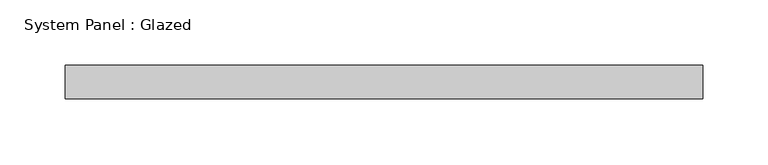
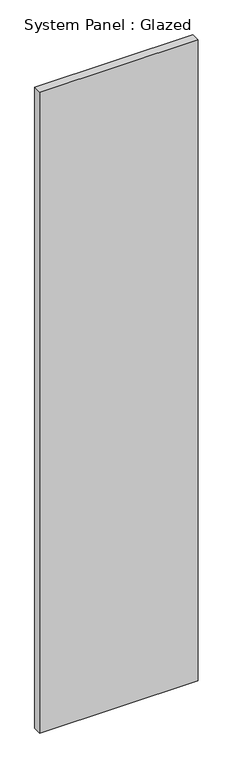
"""IFC4 building model written with IfcOpenShell, lengths in millimetres: plate geometry, System Panel : Glazed."""

from ifc_helpers import new_model, si_unit, origin, origin_with_axes, place, context, project, spatial, polyline, outline, extrude, source, transform, mapped, element, save


def system_panel_glazed_5e4042f1(model_context):
    return source(origin(), model_context, "Body", "SweptSolid", [
        extrude(outline(polyline([(243.5110562, -44.45), (-243.5110562, -44.45), (-243.5110562, -19.05), (243.5110562, -19.05), (243.5110562, -44.45)])), origin_with_axes(), (0.0, 0.0, 1.0), 2082.8),
    ])


if __name__ == "__main__":
    model = new_model("IFC4")
    model_context = context("Model", 3, world=origin())
    ifc_project = project(units=[si_unit("LENGTHUNIT", "METRE", prefix="MILLI")], contexts=[model_context])
    site = spatial("IfcSite", under=ifc_project)
    building = spatial("IfcBuilding", under=site)
    placement = place(None, origin())
    system_panel_glazed_shape = system_panel_glazed_5e4042f1(model_context)
    element("IfcPlate", 1, ObjectType="System Panel : Glazed", at=placement, inside=building, context=model_context, shape_type="MappedRepresentation", body=[
        mapped(system_panel_glazed_shape, transform((0.0, 0.0, 0.0), x_axis=(1.0, 0.0, 0.0), y_axis=(0.0, 1.0, 0.0), z_axis=(0.0, 0.0, 1.0))),
    ])
    save(model, "model.ifc")

# Revit data of these elements
# Type "System Panel : Glazed"
#   Construction Type Id = "GSP4R"
#   Analytic Construction = "1/8 in Pilkington single glazing"
#   Visual Light Transmittance = 0.9
#   Solar Heat Gain Coefficient = 0.86
#   Heat Transfer Coefficient (U) = 1.18115 BTU/(h·ft²·°F)
#   Define Thermal Properties by = 1
# Element 1 (IfcPlate, "System Panel : Glazed")
#   Materials on its faces: "Glass"
# Materials
#   "Glass": class "Glass", colour RGB 0 128 192, transparency 0.75, Description = "Soda Lime Glass", Cost = 0
